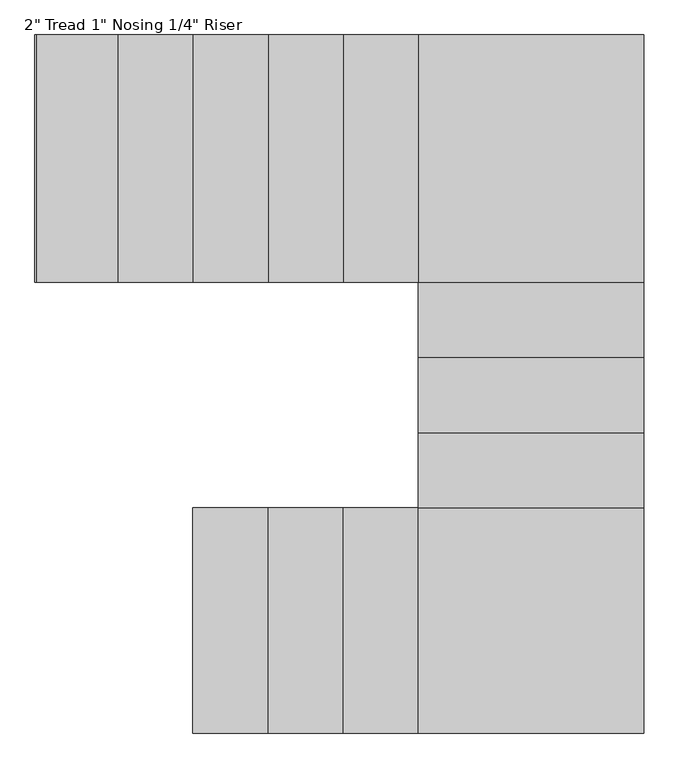
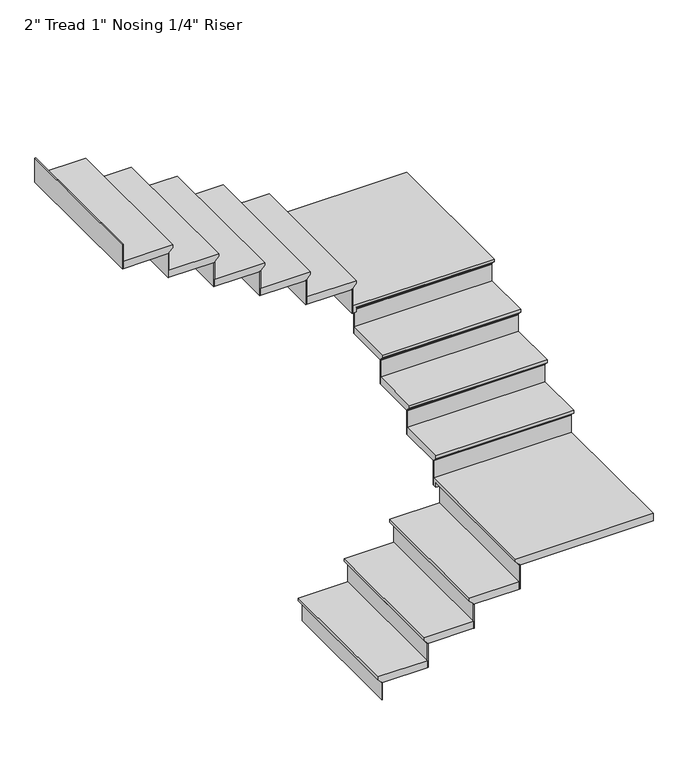
"""IFC4 building model written with IfcOpenShell, lengths in millimetres: stair flight geometry."""

from ifc_helpers import new_model, si_unit, origin, place, context, project, spatial, faceted_brep, source, transform, mapped, element, save


def stair_flight_961aca31(model_context):
    return source(origin(), model_context, "Body", "Brep", [
        faceted_brep([(938.5174794, -182.0870507, 6551.0833333), (938.5174794, -182.0870507, 6570.1333333), (938.5174794, 732.3129493, 6570.1333333), (938.5174794, 732.3129493, 6551.0833333), (963.9174794, -182.0870507, 6525.6833333), (963.9174794, 732.3129493, 6525.6833333), (1268.7174794, -182.0870507, 6570.1333333), (1268.7174794, 732.3129493, 6570.1333333), (963.9174794, 732.3129493, 6519.3333333), (1268.7174794, 732.3129493, 6519.3333333), (1268.7174794, -182.0870507, 6519.3333333), (963.9174794, -182.0870507, 6519.3333333)], [[[0, 1, 2, 3]], [[4, 0, 3, 5]], [[2, 1, 6, 7]], [[8, 9, 10, 11]], [[2, 7, 9, 8, 5, 3]], [[8, 11, 4, 5]], [[6, 1, 0, 4, 11, 10]], [[7, 6, 10, 9]]]),
        faceted_brep([(963.9174794, -182.0870507, 6519.3333333), (963.9174794, -182.0870507, 6400.8), (970.2674794, -182.0870507, 6400.8), (970.2674794, -182.0870507, 6519.3333333), (963.9174794, 732.3129493, 6519.3333333), (970.2674794, 732.3129493, 6519.3333333), (970.2674794, 732.3129493, 6400.8), (963.9174794, 732.3129493, 6400.8)], [[[0, 1, 2, 3]], [[4, 5, 6, 7]], [[1, 0, 4, 7]], [[2, 1, 7, 6]], [[3, 2, 6, 5]], [[0, 3, 5, 4]]]),
        faceted_brep([(1268.7174794, -182.0870507, 6688.6666667), (1268.7174794, -182.0870507, 6519.3333333), (1275.0674794, -182.0870507, 6519.3333333), (1275.0674794, -182.0870507, 6688.6666667), (1268.7174794, 732.3129493, 6688.6666667), (1275.0674794, 732.3129493, 6688.6666667), (1275.0674794, 732.3129493, 6519.3333333), (1268.7174794, 732.3129493, 6519.3333333)], [[[0, 1, 2, 3]], [[4, 5, 6, 7]], [[1, 0, 4, 7]], [[2, 1, 7, 6]], [[3, 2, 6, 5]], [[0, 3, 5, 4]]]),
        faceted_brep([(1243.3174794, 732.3129493, 6739.4666667), (1243.3174794, -182.0870507, 6739.4666667), (1573.5174794, -182.0870507, 6739.4666667), (1573.5174794, 732.3129493, 6739.4666667), (1268.7174794, 732.3129493, 6688.6666667), (1573.5174794, 732.3129493, 6688.6666667), (1573.5174794, -182.0870507, 6688.6666667), (1268.7174794, -182.0870507, 6688.6666667), (1268.7174794, 732.3129493, 6695.0166667), (1243.3174794, 732.3129493, 6720.4166667), (1268.7174794, -182.0870507, 6695.0166667), (1243.3174794, -182.0870507, 6720.4166667)], [[[0, 1, 2, 3]], [[4, 5, 6, 7]], [[0, 3, 5, 4, 8, 9]], [[4, 7, 10, 8]], [[2, 1, 11, 10, 7, 6]], [[3, 2, 6, 5]], [[11, 1, 0, 9]], [[10, 11, 9, 8]]]),
        faceted_brep([(1573.5174794, -182.0870507, 6858.0), (1573.5174794, -182.0870507, 6688.6666667), (1579.8674794, -182.0870507, 6688.6666667), (1579.8674794, -182.0870507, 6858.0), (1573.5174794, 732.3129493, 6858.0), (1579.8674794, 732.3129493, 6858.0), (1579.8674794, 732.3129493, 6688.6666667), (1573.5174794, 732.3129493, 6688.6666667)], [[[0, 1, 2, 3]], [[4, 5, 6, 7]], [[1, 0, 4, 7]], [[2, 1, 7, 6]], [[3, 2, 6, 5]], [[0, 3, 5, 4]]]),
        faceted_brep([(1548.1174794, 732.3129493, 6908.8), (1548.1174794, -182.0870507, 6908.8), (1878.3174794, -182.0870507, 6908.8), (1878.3174794, 732.3129493, 6908.8), (1573.5174794, 732.3129493, 6858.0), (1878.3174794, 732.3129493, 6858.0), (1878.3174794, -182.0870507, 6858.0), (1573.5174794, -182.0870507, 6858.0), (1573.5174794, 732.3129493, 6864.35), (1548.1174794, 732.3129493, 6889.75), (1573.5174794, -182.0870507, 6864.35), (1548.1174794, -182.0870507, 6889.75)], [[[0, 1, 2, 3]], [[4, 5, 6, 7]], [[0, 3, 5, 4, 8, 9]], [[4, 7, 10, 8]], [[2, 1, 11, 10, 7, 6]], [[3, 2, 6, 5]], [[11, 1, 0, 9]], [[10, 11, 9, 8]]]),
        faceted_brep([(1878.3174794, -182.0870507, 7027.3333333), (1878.3174794, -182.0870507, 6858.0), (1884.6674794, -182.0870507, 6858.0), (1884.6674794, -182.0870507, 7027.3333333), (1878.3174794, 732.3129493, 7027.3333333), (1884.6674794, 732.3129493, 7027.3333333), (1884.6674794, 732.3129493, 6858.0), (1878.3174794, 732.3129493, 6858.0)], [[[0, 1, 2, 3]], [[4, 5, 6, 7]], [[1, 0, 4, 7]], [[2, 1, 7, 6]], [[3, 2, 6, 5]], [[0, 3, 5, 4]]]),
        faceted_brep([(2767.3174794, -182.0870507, 7078.1333333), (2767.3174794, 757.7129493, 7078.1333333), (1852.9174794, 757.7129493, 7078.1333333), (1852.9174794, -182.0870507, 7078.1333333), (1852.9174794, 732.3129493, 7027.3333333), (1852.9174794, 757.7129493, 7027.3333333), (2767.3174794, 757.7129493, 7027.3333333), (2767.3174794, -182.0870507, 7027.3333333), (1878.3174794, -182.0870507, 7027.3333333), (1878.3174794, 732.3129493, 7027.3333333), (1852.9174794, 732.3129493, 7059.0833333), (1852.9174794, -182.0870507, 7059.0833333), (1878.3174794, 732.3129493, 7033.6833333), (1878.3174794, -182.0870507, 7033.6833333)], [[[0, 1, 2, 3]], [[4, 5, 6, 7, 8, 9]], [[3, 2, 5, 4, 10, 11]], [[4, 9, 12, 10]], [[9, 8, 13, 12]], [[0, 3, 11, 13, 8, 7]], [[1, 0, 7, 6]], [[2, 1, 6, 5]], [[13, 11, 10, 12]]]),
        faceted_brep([(2767.3174794, 757.7129493, 7196.6666667), (2767.3174794, 757.7129493, 7027.3333333), (2767.3174794, 764.0629493, 7027.3333333), (2767.3174794, 764.0629493, 7196.6666667), (1852.9174794, 757.7129493, 7196.6666667), (1852.9174794, 764.0629493, 7196.6666667), (1852.9174794, 764.0629493, 7027.3333333), (1852.9174794, 757.7129493, 7027.3333333)], [[[0, 1, 2, 3]], [[4, 5, 6, 7]], [[1, 0, 4, 7]], [[2, 1, 7, 6]], [[3, 2, 6, 5]], [[0, 3, 5, 4]]]),
        faceted_brep([(1852.9174794, 732.3129493, 7247.4666667), (2767.3174794, 732.3129493, 7247.4666667), (2767.3174794, 1062.5129493, 7247.4666667), (1852.9174794, 1062.5129493, 7247.4666667), (1852.9174794, 757.7129493, 7196.6666667), (1852.9174794, 1062.5129493, 7196.6666667), (2767.3174794, 1062.5129493, 7196.6666667), (2767.3174794, 757.7129493, 7196.6666667), (1852.9174794, 757.7129493, 7203.0166667), (1852.9174794, 732.3129493, 7228.4166667), (2767.3174794, 757.7129493, 7203.0166667), (2767.3174794, 732.3129493, 7228.4166667)], [[[0, 1, 2, 3]], [[4, 5, 6, 7]], [[0, 3, 5, 4, 8, 9]], [[4, 7, 10, 8]], [[2, 1, 11, 10, 7, 6]], [[3, 2, 6, 5]], [[11, 1, 0, 9]], [[10, 11, 9, 8]]]),
        faceted_brep([(2767.3174794, 1062.5129493, 7366.0), (2767.3174794, 1062.5129493, 7196.6666667), (2767.3174794, 1068.8629493, 7196.6666667), (2767.3174794, 1068.8629493, 7366.0), (1852.9174794, 1062.5129493, 7366.0), (1852.9174794, 1068.8629493, 7366.0), (1852.9174794, 1068.8629493, 7196.6666667), (1852.9174794, 1062.5129493, 7196.6666667)], [[[0, 1, 2, 3]], [[4, 5, 6, 7]], [[1, 0, 4, 7]], [[2, 1, 7, 6]], [[3, 2, 6, 5]], [[0, 3, 5, 4]]]),
        faceted_brep([(1852.9174794, 1037.1129493, 7416.8), (2767.3174794, 1037.1129493, 7416.8), (2767.3174794, 1367.3129493, 7416.8), (1852.9174794, 1367.3129493, 7416.8), (1852.9174794, 1062.5129493, 7366.0), (1852.9174794, 1367.3129493, 7366.0), (2767.3174794, 1367.3129493, 7366.0), (2767.3174794, 1062.5129493, 7366.0), (1852.9174794, 1062.5129493, 7372.35), (1852.9174794, 1037.1129493, 7397.75), (2767.3174794, 1062.5129493, 7372.35), (2767.3174794, 1037.1129493, 7397.75)], [[[0, 1, 2, 3]], [[4, 5, 6, 7]], [[0, 3, 5, 4, 8, 9]], [[4, 7, 10, 8]], [[2, 1, 11, 10, 7, 6]], [[3, 2, 6, 5]], [[11, 1, 0, 9]], [[10, 11, 9, 8]]]),
        faceted_brep([(2767.3174794, 1367.3129493, 7535.3333333), (2767.3174794, 1367.3129493, 7366.0), (2767.3174794, 1373.6629493, 7366.0), (2767.3174794, 1373.6629493, 7535.3333333), (1852.9174794, 1367.3129493, 7535.3333333), (1852.9174794, 1373.6629493, 7535.3333333), (1852.9174794, 1373.6629493, 7366.0), (1852.9174794, 1367.3129493, 7366.0)], [[[0, 1, 2, 3]], [[4, 5, 6, 7]], [[1, 0, 4, 7]], [[2, 1, 7, 6]], [[3, 2, 6, 5]], [[0, 3, 5, 4]]]),
        faceted_brep([(1852.9174794, 1341.9129493, 7586.1333333), (2767.3174794, 1341.9129493, 7586.1333333), (2767.3174794, 1672.1129493, 7586.1333333), (1852.9174794, 1672.1129493, 7586.1333333), (1852.9174794, 1367.3129493, 7535.3333333), (1852.9174794, 1672.1129493, 7535.3333333), (2767.3174794, 1672.1129493, 7535.3333333), (2767.3174794, 1367.3129493, 7535.3333333), (1852.9174794, 1367.3129493, 7541.6833333), (1852.9174794, 1341.9129493, 7567.0833333), (2767.3174794, 1367.3129493, 7541.6833333), (2767.3174794, 1341.9129493, 7567.0833333)], [[[0, 1, 2, 3]], [[4, 5, 6, 7]], [[0, 3, 5, 4, 8, 9]], [[4, 7, 10, 8]], [[2, 1, 11, 10, 7, 6]], [[3, 2, 6, 5]], [[11, 1, 0, 9]], [[10, 11, 9, 8]]]),
        faceted_brep([(2767.3174794, 1672.1129493, 7704.6666667), (2767.3174794, 1672.1129493, 7535.3333333), (2767.3174794, 1678.4629493, 7535.3333333), (2767.3174794, 1678.4629493, 7704.6666667), (1852.9174794, 1672.1129493, 7704.6666667), (1852.9174794, 1678.4629493, 7704.6666667), (1852.9174794, 1678.4629493, 7535.3333333), (1852.9174794, 1672.1129493, 7535.3333333)], [[[0, 1, 2, 3]], [[4, 5, 6, 7]], [[1, 0, 4, 7]], [[2, 1, 7, 6]], [[3, 2, 6, 5]], [[0, 3, 5, 4]]]),
        faceted_brep([(2767.3174794, 2650.0129493, 7755.4666667), (1827.5174794, 2650.0129493, 7755.4666667), (1827.5174794, 1646.7129493, 7755.4666667), (2767.3174794, 1646.7129493, 7755.4666667), (1852.9174794, 1646.7129493, 7704.6666667), (1827.5174794, 1646.7129493, 7704.6666667), (1827.5174794, 2650.0129493, 7704.6666667), (2767.3174794, 2650.0129493, 7704.6666667), (2767.3174794, 1672.1129493, 7704.6666667), (1852.9174794, 1672.1129493, 7704.6666667), (1852.9174794, 1646.7129493, 7736.4166667), (2767.3174794, 1646.7129493, 7736.4166667), (1852.9174794, 1672.1129493, 7711.0166667), (2767.3174794, 1672.1129493, 7711.0166667)], [[[0, 1, 2, 3]], [[4, 5, 6, 7, 8, 9]], [[3, 2, 5, 4, 10, 11]], [[4, 9, 12, 10]], [[9, 8, 13, 12]], [[0, 3, 11, 13, 8, 7]], [[1, 0, 7, 6]], [[2, 1, 6, 5]], [[13, 11, 10, 12]]]),
        faceted_brep([(1827.5174794, 2650.0129493, 7874.0), (1827.5174794, 2650.0129493, 7704.6666667), (1821.1674794, 2650.0129493, 7704.6666667), (1821.1674794, 2650.0129493, 7874.0), (1827.5174794, 1646.7129493, 7874.0), (1821.1674794, 1646.7129493, 7874.0), (1821.1674794, 1646.7129493, 7704.6666667), (1827.5174794, 1646.7129493, 7704.6666667)], [[[0, 1, 2, 3]], [[4, 5, 6, 7]], [[1, 0, 4, 7]], [[2, 1, 7, 6]], [[3, 2, 6, 5]], [[0, 3, 5, 4]]]),
        faceted_brep([(1852.9174794, 1646.7129493, 7924.8), (1852.9174794, 2650.0129493, 7924.8), (1522.7174794, 2650.0129493, 7924.8), (1522.7174794, 1646.7129493, 7924.8), (1827.5174794, 1646.7129493, 7874.0), (1522.7174794, 1646.7129493, 7874.0), (1522.7174794, 2650.0129493, 7874.0), (1827.5174794, 2650.0129493, 7874.0), (1827.5174794, 1646.7129493, 7880.35), (1852.9174794, 1646.7129493, 7905.75), (1827.5174794, 2650.0129493, 7880.35), (1852.9174794, 2650.0129493, 7905.75)], [[[0, 1, 2, 3]], [[4, 5, 6, 7]], [[0, 3, 5, 4, 8, 9]], [[4, 7, 10, 8]], [[2, 1, 11, 10, 7, 6]], [[3, 2, 6, 5]], [[11, 1, 0, 9]], [[10, 11, 9, 8]]]),
        faceted_brep([(1522.7174794, 2650.0129493, 8043.3333333), (1522.7174794, 2650.0129493, 7874.0), (1516.3674794, 2650.0129493, 7874.0), (1516.3674794, 2650.0129493, 8043.3333333), (1522.7174794, 1646.7129493, 8043.3333333), (1516.3674794, 1646.7129493, 8043.3333333), (1516.3674794, 1646.7129493, 7874.0), (1522.7174794, 1646.7129493, 7874.0)], [[[0, 1, 2, 3]], [[4, 5, 6, 7]], [[1, 0, 4, 7]], [[2, 1, 7, 6]], [[3, 2, 6, 5]], [[0, 3, 5, 4]]]),
        faceted_brep([(1548.1174794, 1646.7129493, 8094.1333333), (1548.1174794, 2650.0129493, 8094.1333333), (1217.9174794, 2650.0129493, 8094.1333333), (1217.9174794, 1646.7129493, 8094.1333333), (1522.7174794, 1646.7129493, 8043.3333333), (1217.9174794, 1646.7129493, 8043.3333333), (1217.9174794, 2650.0129493, 8043.3333333), (1522.7174794, 2650.0129493, 8043.3333333), (1522.7174794, 1646.7129493, 8049.6833333), (1548.1174794, 1646.7129493, 8075.0833333), (1522.7174794, 2650.0129493, 8049.6833333), (1548.1174794, 2650.0129493, 8075.0833333)], [[[0, 1, 2, 3]], [[4, 5, 6, 7]], [[0, 3, 5, 4, 8, 9]], [[4, 7, 10, 8]], [[2, 1, 11, 10, 7, 6]], [[3, 2, 6, 5]], [[11, 1, 0, 9]], [[10, 11, 9, 8]]]),
        faceted_brep([(1217.9174794, 2650.0129493, 8212.6666667), (1217.9174794, 2650.0129493, 8043.3333333), (1211.5674794, 2650.0129493, 8043.3333333), (1211.5674794, 2650.0129493, 8212.6666667), (1217.9174794, 1646.7129493, 8212.6666667), (1211.5674794, 1646.7129493, 8212.6666667), (1211.5674794, 1646.7129493, 8043.3333333), (1217.9174794, 1646.7129493, 8043.3333333)], [[[0, 1, 2, 3]], [[4, 5, 6, 7]], [[1, 0, 4, 7]], [[2, 1, 7, 6]], [[3, 2, 6, 5]], [[0, 3, 5, 4]]]),
        faceted_brep([(1243.3174794, 1646.7129493, 8263.4666667), (1243.3174794, 2650.0129493, 8263.4666667), (913.1174794, 2650.0129493, 8263.4666667), (913.1174794, 1646.7129493, 8263.4666667), (1217.9174794, 1646.7129493, 8212.6666667), (913.1174794, 1646.7129493, 8212.6666667), (913.1174794, 2650.0129493, 8212.6666667), (1217.9174794, 2650.0129493, 8212.6666667), (1217.9174794, 1646.7129493, 8219.0166667), (1243.3174794, 1646.7129493, 8244.4166667), (1217.9174794, 2650.0129493, 8219.0166667), (1243.3174794, 2650.0129493, 8244.4166667)], [[[0, 1, 2, 3]], [[4, 5, 6, 7]], [[0, 3, 5, 4, 8, 9]], [[4, 7, 10, 8]], [[2, 1, 11, 10, 7, 6]], [[3, 2, 6, 5]], [[11, 1, 0, 9]], [[10, 11, 9, 8]]]),
        faceted_brep([(913.1174794, 2650.0129493, 8382.0), (913.1174794, 2650.0129493, 8212.6666667), (906.7674794, 2650.0129493, 8212.6666667), (906.7674794, 2650.0129493, 8382.0), (913.1174794, 1646.7129493, 8382.0), (906.7674794, 1646.7129493, 8382.0), (906.7674794, 1646.7129493, 8212.6666667), (913.1174794, 1646.7129493, 8212.6666667)], [[[0, 1, 2, 3]], [[4, 5, 6, 7]], [[1, 0, 4, 7]], [[2, 1, 7, 6]], [[3, 2, 6, 5]], [[0, 3, 5, 4]]]),
        faceted_brep([(938.5174794, 1646.7129493, 8432.8), (938.5174794, 2650.0129493, 8432.8), (608.3174794, 2650.0129493, 8432.8), (608.3174794, 1646.7129493, 8432.8), (913.1174794, 1646.7129493, 8382.0), (608.3174794, 1646.7129493, 8382.0), (608.3174794, 2650.0129493, 8382.0), (913.1174794, 2650.0129493, 8382.0), (913.1174794, 1646.7129493, 8388.35), (938.5174794, 1646.7129493, 8413.75), (913.1174794, 2650.0129493, 8388.35), (938.5174794, 2650.0129493, 8413.75)], [[[0, 1, 2, 3]], [[4, 5, 6, 7]], [[0, 3, 5, 4, 8, 9]], [[4, 7, 10, 8]], [[2, 1, 11, 10, 7, 6]], [[3, 2, 6, 5]], [[11, 1, 0, 9]], [[10, 11, 9, 8]]]),
        faceted_brep([(608.3174794, 2650.0129493, 8551.3333333), (608.3174794, 2650.0129493, 8382.0), (601.9674794, 2650.0129493, 8382.0), (601.9674794, 2650.0129493, 8551.3333333), (608.3174794, 1646.7129493, 8551.3333333), (601.9674794, 1646.7129493, 8551.3333333), (601.9674794, 1646.7129493, 8382.0), (608.3174794, 1646.7129493, 8382.0)], [[[0, 1, 2, 3]], [[4, 5, 6, 7]], [[1, 0, 4, 7]], [[2, 1, 7, 6]], [[3, 2, 6, 5]], [[0, 3, 5, 4]]]),
        faceted_brep([(303.5174794, 2650.0129493, 8720.6666667), (303.5174794, 2650.0129493, 8551.3333333), (297.1674794, 2650.0129493, 8551.3333333), (297.1674794, 2650.0129493, 8720.6666667), (303.5174794, 1646.7129493, 8720.6666667), (297.1674794, 1646.7129493, 8720.6666667), (297.1674794, 1646.7129493, 8551.3333333), (303.5174794, 1646.7129493, 8551.3333333)], [[[0, 1, 2, 3]], [[4, 5, 6, 7]], [[1, 0, 4, 7]], [[2, 1, 7, 6]], [[3, 2, 6, 5]], [[0, 3, 5, 4]]]),
        faceted_brep([(633.7174794, 1646.7129493, 8602.1333333), (633.7174794, 2650.0129493, 8602.1333333), (303.5174794, 2650.0129493, 8602.1333333), (303.5174794, 1646.7129493, 8602.1333333), (608.3174794, 1646.7129493, 8551.3333333), (303.5174794, 1646.7129493, 8551.3333333), (303.5174794, 2650.0129493, 8551.3333333), (608.3174794, 2650.0129493, 8551.3333333), (608.3174794, 1646.7129493, 8557.6833333), (633.7174794, 1646.7129493, 8583.0833333), (608.3174794, 2650.0129493, 8557.6833333), (633.7174794, 2650.0129493, 8583.0833333)], [[[0, 1, 2, 3]], [[4, 5, 6, 7]], [[0, 3, 5, 4, 8, 9]], [[4, 7, 10, 8]], [[2, 1, 11, 10, 7, 6]], [[3, 2, 6, 5]], [[11, 1, 0, 9]], [[10, 11, 9, 8]]]),
    ])


if __name__ == "__main__":
    model = new_model("IFC4")
    model_context = context("Model", 3, world=origin())
    ifc_project = project(units=[si_unit("LENGTHUNIT", "METRE", prefix="MILLI")], contexts=[model_context])
    site = spatial("IfcSite", under=ifc_project)
    building = spatial("IfcBuilding", under=site)
    placement = place(None, origin())
    stair_flight_shape = stair_flight_961aca31(model_context)
    element("IfcStairFlight", 1, ObjectType="2\" Tread 1\" Nosing 1/4\" Riser", at=placement, inside=building, context=model_context, shape_type="MappedRepresentation", body=[
        mapped(stair_flight_shape, transform((0.0, 0.0, 0.0), x_axis=(1.0, 0.0, 0.0), y_axis=(0.0, 1.0, 0.0), z_axis=(0.0, 0.0, 1.0))),
    ])
    save(model, "model.ifc")
